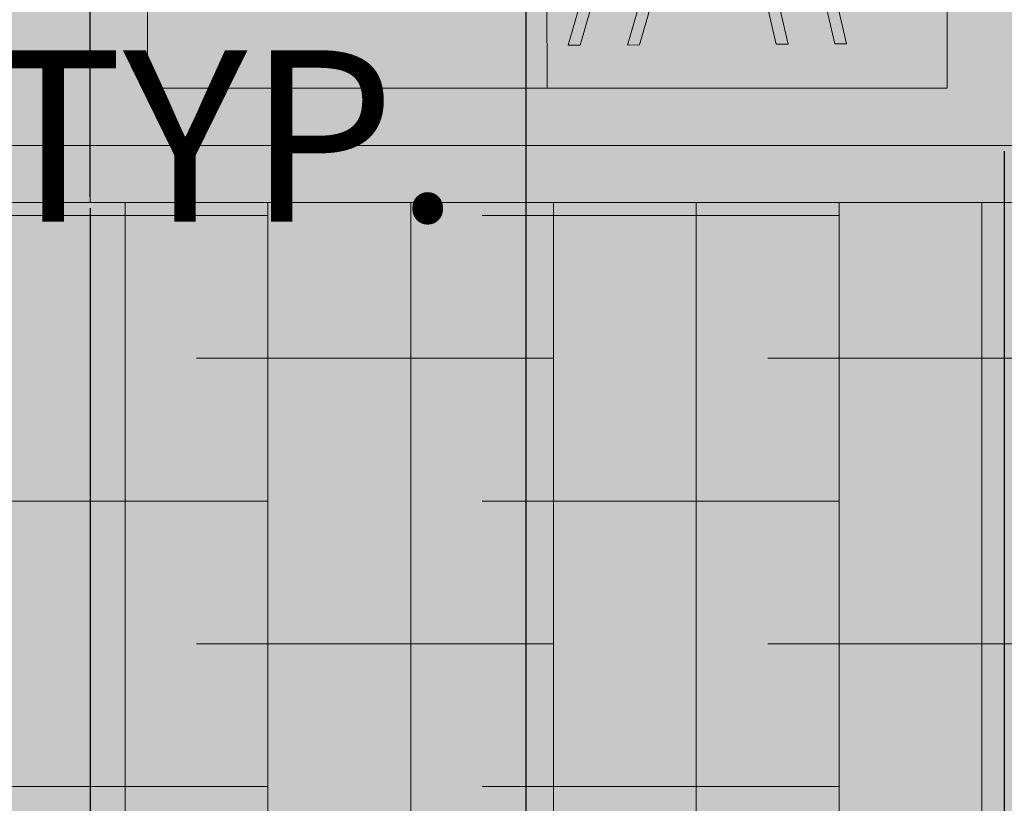
# Model space of a CAD drawing. Units: millimetres. Extents: x 11032 to 26788, y 3406 to 24505.
# Tile 5 of 78: x 16283 to 17145, y 6736 to 7421. Entities that reach past the tile are written whole.
import ezdxf

# ---------------------------------------------------------------- set-up
doc = ezdxf.new("R2010")
doc.units = ezdxf.units.MM
doc.header["$MEASUREMENT"] = 0
for name, color, linetype, lineweight in [('A-ANNO-DIMS', 2, 'Continuous', 18), ('A-FURN', 8, 'Continuous', 13), ('A-FURN-PATT', 8, 'Continuous', 13), ('A-GLAZ', 250, 'Continuous', 20), ('A-WALL-INTR', 8, 'Continuous', 18), ('A-WALL-PLIN-PATT', 253, 'Continuous', 13)]:
    doc.layers.add(name, color=color, linetype=linetype, lineweight=lineweight)
doc.layers.add('A-GLAZ-FRAM-PATT', color=250, linetype='Continuous', lineweight=13, true_color=0x262627)
doc.layers.add('A-WALL-INTR-PATT', color=251, linetype='Continuous', lineweight=13, true_color=0x6c6b6a)
doc.styles.get("Standard").update_dxf_attribs({"font": 'arial.ttf'})
doc.dimstyles.get("Standard").update_dxf_attribs({"dimtxt": 150, "dimasz": 100, "dimexe": 10, "dimexo": 5, "dimgap": 5, "dimtad": 0, "dimtih": 1, "dimtoh": 1, "dimdec": 0, "dimzin": 0, "dimdsep": 46, "dimtxsty": 'Standard', "dimcen": 0.09, "dimadec": 0, "dimazin": 0, "dimtfac": 1, "dimtdec": 0, "dimtofl": 0, "dimtmove": 0, "dimatfit": 3, "dimfxl": 1, "dimtolj": 1, "dimtzin": 0, "dimarcsym": 0})

# ---------------------------------------------------------------- blocks, each defined once
blk = doc.blocks.new('DINING-CHAIR-ELEV')
blk.add_line((228.68, 123.43), (51.04, 132.61))
for points in [[(0, 379.55), (49.45, 435.94), (114.12, 434.53)], [(61.18, 132.09), (30.79, 1.16), (20.53, 1.21), (59.55, 169.26), (0, 379.55), (61.9, 377.89)], [(111.9, 129.47), (82.06, 0.91), (71.8, 0.96), (101.76, 129.99)], [(165.28, 126.71), (201.76, 0.31), (212.19, 0.26), (175.85, 126.16)]]:
    blk.add_lwpolyline(points)
for points in [[(218.11, 123.98), (253.88, 0.05), (264.3, 0), (228.68, 123.43), (238.32, 182.18, 0.148451), (167.47, 178.33), (96.61, 174.48, 0.097012), (61.9, 377.89), (114.12, 434.53, -0.154833), (167.82, 178.46)], [(132.04, 176.4, 0.156877), (88.01, 406.21), (24.72, 407.74)]]:
    blk.add_lwpolyline(points, format="xyb")
blk = doc.blocks.new('*D16')
at = {"layer": 'A-ANNO-DIMS', "color": 0, "lineweight": -2, "transparency": 16777216}
for p, q in [((15741.74, 7821.05), (15812.13, 7821.05)), ((15802.13, 7721.05), (15802.13, 7685.69)), ((15802.13, 7485.11), (15802.13, 7520.47)), ((15741.74, 7385.11), (15812.13, 7385.11))]:
    blk.add_line(p, q, dxfattribs=at)
at = {"layer": 'A-ANNO-DIMS', "color": 0, "transparency": 16777216}
for points in [[(15785.47, 7721.05), (15818.8, 7721.05), (15802.13, 7821.05)], [(15785.47, 7485.11), (15818.8, 7485.11), (15802.13, 7385.11)]]:
    blk.add_solid(points, dxfattribs=at)
at = {"layer": 'Defpoints', "color": 0, "transparency": 16777216}
for p in [(15736.74, 7821.05), (15802.13, 7821.05), (15736.74, 7385.11)]:
    blk.add_point(p, dxfattribs=at)
at = {"layer": 'A-ANNO-DIMS', "color": 0, "transparency": 16777216, "insert": (15802.13, 7603.08), "char_height": 150, "attachment_point": 5}
blk.add_mtext('\\A1;CHAIR 436 TYP.', dxfattribs=at)
blk = doc.blocks.new('*D17')
at = {"layer": 'A-ANNO-DIMS', "color": 0, "lineweight": -2, "transparency": 16777216}
for p, q in [((15472.44, 7380.11), (15472.44, 7309.72)), ((15736.74, 7380.11), (15736.74, 7309.72)), ((15572.44, 7319.72), (15636.74, 7319.72)), ((15736.74, 7319.72), (15836.74, 7319.72))]:
    blk.add_line(p, q, dxfattribs=at)
at = {"layer": 'A-ANNO-DIMS', "color": 0, "transparency": 16777216}
for points in [[(15572.44, 7336.38), (15572.44, 7303.05), (15472.44, 7319.72)], [(15636.74, 7336.38), (15636.74, 7303.05), (15736.74, 7319.72)]]:
    blk.add_solid(points, dxfattribs=at)
at = {"layer": 'Defpoints', "color": 0, "transparency": 16777216}
for p in [(15472.44, 7385.11), (15736.74, 7385.11), (15736.74, 7319.72)]:
    blk.add_point(p, dxfattribs=at)
at = {"layer": 'A-ANNO-DIMS', "color": 0, "transparency": 16777216, "insert": (16266.37, 7319.72), "char_height": 150, "attachment_point": 5}
blk.add_mtext('\\A1;264 TYP.', dxfattribs=at)
blk = doc.blocks.new('*D36')
at = {"layer": 'A-ANNO-DIMS', "color": 0, "lineweight": -2, "transparency": 16777216}
for p, q in [((12301.26, 17115.89), (12301.26, 24416.86)), ((25397.4, 4466.4), (25397.4, 24416.86)), ((12401.26, 24406.86), (18569.2, 24406.86)), ((25297.4, 24406.86), (19129.47, 24406.86))]:
    blk.add_line(p, q, dxfattribs=at)
at = {"layer": 'A-ANNO-DIMS', "color": 0, "transparency": 16777216}
for points in [[(12401.26, 24423.52), (12401.26, 24390.19), (12301.26, 24406.86)], [(25297.4, 24423.52), (25297.4, 24390.19), (25397.4, 24406.86)]]:
    blk.add_solid(points, dxfattribs=at)
at = {"layer": 'Defpoints', "color": 0, "transparency": 16777216}
for p in [(25397.4, 24406.86), (12301.26, 17110.89), (25397.4, 4461.4)]:
    blk.add_point(p, dxfattribs=at)
at = {"layer": 'A-ANNO-DIMS', "color": 0, "transparency": 16777216, "insert": (18849.33, 24406.86), "char_height": 150, "attachment_point": 5}
blk.add_mtext('\\A1;13096', dxfattribs=at)
blk = doc.blocks.new('*D37')
at = {"layer": 'A-ANNO-DIMS', "color": 0, "lineweight": -2, "transparency": 16777216}
for p, q in [((18087.74, 23450.36), (11334.76, 23450.36)), ((11344.76, 23350.36), (11344.76, 14037.46)), ((11344.76, 4561.4), (11344.76, 13874.29)), ((12927.66, 4461.4), (11334.76, 4461.4))]:
    blk.add_line(p, q, dxfattribs=at)
at = {"layer": 'A-ANNO-DIMS', "color": 0, "transparency": 16777216}
for points in [[(11328.1, 23350.36), (11361.43, 23350.36), (11344.76, 23450.36)], [(11328.1, 4561.4), (11361.43, 4561.4), (11344.76, 4461.4)]]:
    blk.add_solid(points, dxfattribs=at)
at = {"layer": 'Defpoints', "color": 0, "transparency": 16777216}
for p in [(11344.76, 23450.36), (18092.74, 23450.36), (12932.66, 4461.4)]:
    blk.add_point(p, dxfattribs=at)
at = {"layer": 'A-ANNO-DIMS', "color": 0, "transparency": 16777216, "insert": (11344.76, 13955.88), "char_height": 150, "attachment_point": 5}
blk.add_mtext('\\A1;18989', dxfattribs=at)
blk = doc.blocks.new('*D49')
at = {"layer": 'A-ANNO-DIMS', "color": 0, "lineweight": -2, "transparency": 16777216}
for p, q in [((17953.45, 10206.41), (17953.45, 3494.9)), ((14996.4, 6406.4), (14996.4, 3494.9)), ((15096.4, 3504.9), (16244.67, 3504.9)), ((17853.45, 3504.9), (16705.18, 3504.9))]:
    blk.add_line(p, q, dxfattribs=at)
at = {"layer": 'A-ANNO-DIMS', "color": 0, "transparency": 16777216}
for points in [[(15096.4, 3521.57), (15096.4, 3488.23), (14996.4, 3504.9)], [(17853.45, 3521.57), (17853.45, 3488.23), (17953.45, 3504.9)]]:
    blk.add_solid(points, dxfattribs=at)
at = {"layer": 'Defpoints', "color": 0, "transparency": 16777216}
for p in [(17953.45, 10211.41), (14996.4, 6411.4), (17953.45, 3504.9)]:
    blk.add_point(p, dxfattribs=at)
at = {"layer": 'A-ANNO-DIMS', "color": 0, "transparency": 16777216, "insert": (16474.93, 3504.9), "char_height": 150, "attachment_point": 5}
blk.add_mtext('\\A1;2957', dxfattribs=at)
blk = doc.blocks.new('*D57')
at = {"layer": 'A-ANNO-DIMS', "color": 0, "lineweight": -2, "transparency": 16777216}
for p, q in [((14994.7, 7266.4), (14994.7, 24416.86)), ((20894.7, 7266.4), (20894.7, 24416.86)), ((15094.7, 24406.86), (17715.98, 24406.86)), ((20794.7, 24406.86), (18173.42, 24406.86))]:
    blk.add_line(p, q, dxfattribs=at)
at = {"layer": 'A-ANNO-DIMS', "color": 0, "transparency": 16777216}
for points in [[(15094.7, 24423.52), (15094.7, 24390.19), (14994.7, 24406.86)], [(20794.7, 24423.52), (20794.7, 24390.19), (20894.7, 24406.86)]]:
    blk.add_solid(points, dxfattribs=at)
at = {"layer": 'Defpoints', "color": 0, "transparency": 16777216}
for p in [(20894.7, 24406.86), (14994.7, 7261.4), (20894.7, 7261.4)]:
    blk.add_point(p, dxfattribs=at)
at = {"layer": 'A-ANNO-DIMS', "color": 0, "transparency": 16777216, "insert": (17944.7, 24406.86), "char_height": 150, "attachment_point": 5}
blk.add_mtext('\\A1;5900', dxfattribs=at)
blk = doc.blocks.new('*D60')
at = {"layer": 'A-ANNO-DIMS', "color": 0, "lineweight": -2, "transparency": 16777216}
for p, q in [((14994.7, 7266.4), (14994.7, 24416.86)), ((16344.7, 7266.4), (16344.7, 24416.86)), ((15094.7, 24406.86), (15448.04, 24406.86)), ((16244.7, 24406.86), (15891.36, 24406.86))]:
    blk.add_line(p, q, dxfattribs=at)
at = {"layer": 'A-ANNO-DIMS', "color": 0, "transparency": 16777216}
for points in [[(15094.7, 24423.52), (15094.7, 24390.19), (14994.7, 24406.86)], [(16244.7, 24423.52), (16244.7, 24390.19), (16344.7, 24406.86)]]:
    blk.add_solid(points, dxfattribs=at)
at = {"layer": 'Defpoints', "color": 0, "transparency": 16777216}
for p in [(16344.7, 24406.86), (14994.7, 7261.4), (16344.7, 7261.4)]:
    blk.add_point(p, dxfattribs=at)
at = {"layer": 'A-ANNO-DIMS', "color": 0, "transparency": 16777216, "insert": (15669.7, 24406.86), "char_height": 150, "attachment_point": 5}
blk.add_mtext('\\A1;1350', dxfattribs=at)
blk = doc.blocks.new('*D61')
at = {"layer": 'A-ANNO-DIMS', "color": 0, "lineweight": -2, "transparency": 16777216}
for p, q in [((17144.7, 7306.4), (17144.7, 3494.9)), ((16344.7, 7256.4), (16344.7, 3494.9)), ((16444.7, 3504.9), (16574.15, 3504.9)), ((17044.7, 3504.9), (16915.26, 3504.9))]:
    blk.add_line(p, q, dxfattribs=at)
at = {"layer": 'A-ANNO-DIMS', "color": 0, "transparency": 16777216}
for points in [[(16444.7, 3521.57), (16444.7, 3488.23), (16344.7, 3504.9)], [(17044.7, 3521.57), (17044.7, 3488.23), (17144.7, 3504.9)]]:
    blk.add_solid(points, dxfattribs=at)
at = {"layer": 'Defpoints', "color": 0, "transparency": 16777216}
for p in [(17144.7, 7311.4), (16344.7, 7261.4), (17144.7, 3504.9)]:
    blk.add_point(p, dxfattribs=at)
at = {"layer": 'A-ANNO-DIMS', "color": 0, "transparency": 16777216, "insert": (16744.7, 3504.9), "char_height": 150, "attachment_point": 5}
blk.add_mtext('\\A1;800', dxfattribs=at)
blk = doc.blocks.new('*D62')
at = {"layer": 'A-ANNO-DIMS', "color": 0, "lineweight": -2, "transparency": 16777216}
for p, q in [((17144.7, 7306.4), (17144.7, 3494.9)), ((17944.7, 7256.4), (17944.7, 3494.9)), ((17244.7, 3504.9), (17374.15, 3504.9)), ((17844.7, 3504.9), (17715.26, 3504.9))]:
    blk.add_line(p, q, dxfattribs=at)
at = {"layer": 'A-ANNO-DIMS', "color": 0, "transparency": 16777216}
for points in [[(17244.7, 3521.57), (17244.7, 3488.23), (17144.7, 3504.9)], [(17844.7, 3521.57), (17844.7, 3488.23), (17944.7, 3504.9)]]:
    blk.add_solid(points, dxfattribs=at)
at = {"layer": 'Defpoints', "color": 0, "transparency": 16777216}
for p in [(17144.7, 7311.4), (17944.7, 7261.4), (17944.7, 3504.9)]:
    blk.add_point(p, dxfattribs=at)
at = {"layer": 'A-ANNO-DIMS', "color": 0, "transparency": 16777216, "insert": (17544.7, 3504.9), "char_height": 150, "attachment_point": 5}
blk.add_mtext('\\A1;800', dxfattribs=at)
blk = doc.blocks.new('*D66')
at = {"layer": 'A-ANNO-DIMS', "color": 0, "lineweight": -2, "transparency": 16777216}
for p, q in [((16725.95, 10296.02), (16725.95, 3494.9)), ((19150.95, 10296.02), (19150.95, 3494.9)), ((16825.95, 3504.9), (17707.63, 3504.9)), ((19050.95, 3504.9), (18169.27, 3504.9))]:
    blk.add_line(p, q, dxfattribs=at)
at = {"layer": 'A-ANNO-DIMS', "color": 0, "transparency": 16777216}
for points in [[(16825.95, 3521.57), (16825.95, 3488.23), (16725.95, 3504.9)], [(19050.95, 3521.57), (19050.95, 3488.23), (19150.95, 3504.9)]]:
    blk.add_solid(points, dxfattribs=at)
at = {"layer": 'Defpoints', "color": 0, "transparency": 16777216}
for p in [(16725.95, 10301.02), (19150.95, 10301.02), (19150.95, 3504.9)]:
    blk.add_point(p, dxfattribs=at)
at = {"layer": 'A-ANNO-DIMS', "color": 0, "transparency": 16777216, "insert": (17938.45, 3504.9), "char_height": 150, "attachment_point": 5}
blk.add_mtext('\\A1;2425', dxfattribs=at)
blk = doc.blocks.new('*D69')
at = {"layer": 'A-ANNO-DIMS', "color": 0, "lineweight": -2, "transparency": 16777216}
for p, q in [((13956.97, 9937.95), (14056.97, 9937.95)), ((14056.97, 9937.95), (15432.5, 8990.95)), ((17944.61, 7261.4), (17944.79, 7261.4)), ((17944.7, 7261.31), (17944.7, 7261.49))]:
    blk.add_line(p, q, dxfattribs=at)
at = {"layer": 'A-ANNO-DIMS', "color": 0, "transparency": 16777216}
blk.add_solid([(15441.95, 9004.68), (15423.05, 8977.22), (15514.87, 8934.24)], dxfattribs=at)
at = {"layer": 'Defpoints', "color": 0, "transparency": 16777216}
for p in [(15514.87, 8934.24), (17944.7, 7261.4)]:
    blk.add_point(p, dxfattribs=at)
at = {"layer": 'A-ANNO-DIMS', "color": 0, "transparency": 16777216, "insert": (13494.04, 9937.95), "char_height": 150, "attachment_point": 5}
blk.add_mtext('\\A1;2X R2950', dxfattribs=at)

msp = doc.modelspace()

# ---------------------------------------------------------------- hatches: boundary and pattern name
at = {"layer": 'A-FURN-PATT'}
h = msp.add_hatch(color=256, dxfattribs=at)
h.set_gradient(color1=(82, 15, 16), color2=(153, 0, 38), name='CURVED')
h.paths.add_polyline_path([(16952.125, 8119), (16926.017, 8147.32, 0.1568775), (16881.989, 7917.509), (16917.415, 7915.583, -0.0970121)], flags=0)
h.paths.add_polyline_path([(16899.908, 8175.64), (16964.58, 8177.046), (17014.03, 8120.657), (16954.484, 7910.365), (16972.017, 7834.84), (16977.75, 7834.965), (17027.199, 7778.576), (16967.653, 7568.284), (17006.665, 7400.238), (16996.411, 7400.187), (16966.016, 7531.114), (16925.439, 7529.018), (16955.395, 7399.983), (16945.141, 7399.932), (16915.295, 7528.494), (16861.916, 7525.736), (16825.435, 7399.337), (16815.012, 7399.285), (16851.35, 7525.19), (16809.087, 7523.007), (16773.319, 7399.078), (16762.896, 7399.026), (16798.521, 7522.461), (16788.882, 7581.207, -0.1476694), (16859.382, 7577.482, -0.1528132), (16911.41, 7830.579), (16902.125, 7870.575), (16848.746, 7867.817), (16830.506, 7804.617), (16830.506, 7793.515), (16827.302, 7793.515), (16812.265, 7741.418), (16801.842, 7741.366), (16816.893, 7793.515), (16775.261, 7793.515), (16760.15, 7741.159), (16749.727, 7741.107), (16764.853, 7793.515), (16650.704, 7793.515), (16662.994, 7750.932), (16652.571, 7750.983), (16640.296, 7793.515), (16598.663, 7793.515), (16610.879, 7751.191), (16600.455, 7751.242), (16588.255, 7793.515), (16490.425, 7793.515), (16480.749, 7751.837), (16470.495, 7751.888), (16480.159, 7793.515), (16443.833, 7793.515, -0.1094051), (16465.746, 7607.731, -0.1476694), (16536.246, 7611.456), (16526.606, 7552.71), (16562.232, 7429.275), (16551.809, 7429.327), (16516.041, 7553.255), (16473.778, 7555.439), (16510.116, 7429.534), (16499.693, 7429.586), (16463.212, 7555.985), (16409.833, 7558.743), (16379.987, 7430.181), (16369.733, 7430.232), (16394.704, 7537.793), (16394.704, 7559.524), (16359.112, 7561.363), (16328.717, 7430.435), (16318.463, 7430.486), (16344.704, 7543.521), (16344.704, 7643.635), (16302.264, 7793.515), (16205.738, 7793.515), (16227.021, 7719.773), (16216.598, 7719.825), (16195.329, 7793.515), (16153.697, 7793.515), (16174.905, 7720.032), (16164.482, 7720.084), (16143.289, 7793.515), (15844.423, 7793.515), (15844.423, 7804.617), (16140.084, 7804.617), (16128.001, 7846.483), (16191.395, 7843.208), (16201.035, 7901.954, 0.1484508), (16130.184, 7898.102), (16059.333, 7894.25, 0.0970121), (16024.622, 8097.666), (16076.839, 8154.307, -0.1548334), (16130.535, 7898.229, -0.1476694), (16201.035, 7901.954), (16191.395, 7843.208), (16202.533, 7804.617), (16299.12, 7804.617), (16297.929, 7808.825), (16347.378, 7865.214), (16412.05, 7863.808, -0.0295496), (16434.494, 7817.915), (16458.237, 7920.19), (16398.691, 8130.481), (16448.141, 8186.871), (16512.813, 8185.465, -0.1548334), (16566.508, 7929.387, -0.1476694), (16637.008, 7933.112), (16627.369, 7874.366), (16647.499, 7804.617), (16742.939, 7804.617), (16741.107, 8264.696), (17994.704, 8264.696), (17994.704, 7796.661), (18112.02, 7796.661), (18134.447, 7874.366), (18124.807, 7933.112, -0.1476694), (18195.307, 7929.387, -0.1548334), (18249.003, 8185.465), (18313.675, 8186.871), (18363.124, 8130.481), (18303.578, 7920.19), (18311.087, 7887.847, -0.0273017), (18332.016, 7930.161), (18396.688, 7931.567), (18446.137, 7875.177), (18423.905, 7796.661), (18470.25, 7796.661), (18470.25, 7785.559), (18420.761, 7785.559), (18386.591, 7664.886), (18425.604, 7496.839), (18415.35, 7496.788), (18384.955, 7627.716), (18344.377, 7625.62), (18374.333, 7496.584), (18364.079, 7496.533), (18334.233, 7625.095), (18280.854, 7622.338), (18244.373, 7495.938), (18233.95, 7495.887), (18270.288, 7621.792), (18228.026, 7619.608), (18192.257, 7495.679), (18181.834, 7495.628), (18217.46, 7619.062), (18207.82, 7677.808, -0.1476694), (18278.32, 7674.083, -0.0514181), (18278.516, 7762.821), (18273.237, 7785.559), (18171.265, 7785.559), (18161.36, 7751.242), (18150.937, 7751.191), (18160.856, 7785.559), (18119.224, 7785.559), (18109.244, 7750.983), (18098.821, 7750.932), (18108.815, 7785.559), (17852.794, 7785.559), (17866.18, 7739.181), (17855.756, 7739.233), (17842.386, 7785.559), (17800.753, 7785.559), (17814.064, 7739.44), (17803.641, 7739.492), (17790.345, 7785.559), (17694.491, 7785.559), (17685.986, 7748.922, -0.0882745), (17728.687, 7746.171), (17719.047, 7687.425), (17754.673, 7563.99), (17744.25, 7564.042), (17708.482, 7687.971), (17666.219, 7690.154), (17702.557, 7564.249), (17692.134, 7564.301), (17655.653, 7690.7), (17602.274, 7693.458), (17572.428, 7564.896), (17562.174, 7564.947), (17592.13, 7693.982), (17551.553, 7696.078), (17521.158, 7565.151), (17510.903, 7565.202), (17549.916, 7733.248), (17535.103, 7785.559), (17484.167, 7785.559), (17484.167, 7796.661), (17531.96, 7796.661), (17490.37, 7943.54), (17539.819, 7999.929), (17604.491, 7998.523, -0.0802486), (17652.289, 7869.096), (17661.422, 7908.439), (17601.876, 8118.731), (17651.326, 8175.12), (17715.998, 8173.714, -0.1548334), (17769.694, 7917.637, -0.1476694), (17840.194, 7921.361), (17830.554, 7862.615), (17849.59, 7796.661), (17894.704, 7796.661), (17894.704, 8239.696), (16741.207, 8239.696), (16742.939, 7804.617), (16768.057, 7804.617), (16785.352, 7864.542), (16775.713, 7923.288, -0.1476694), (16846.212, 7919.563, -0.1548334)], flags=17)
h.paths.add_polyline_path([(16899.908, 8175.64), (16964.58, 8177.046), (17014.03, 8120.657), (16954.484, 7910.365), (16993.496, 7742.318), (16983.242, 7742.267), (16952.847, 7873.195), (16912.27, 7871.099), (16942.225, 7742.064), (16931.971, 7742.013), (16902.125, 7870.575), (16848.746, 7867.817), (16812.265, 7741.418), (16801.842, 7741.366), (16838.181, 7867.271), (16795.918, 7865.087), (16760.15, 7741.159), (16749.727, 7741.107), (16785.352, 7864.542), (16775.713, 7923.288, -0.1476694), (16846.212, 7919.563, -0.1548334)], flags=0)
h.paths.add_polyline_path([(16899.908, 8175.64), (16964.58, 8177.046), (17014.03, 8120.657), (16954.484, 7910.365), (16972.017, 7834.84), (16977.75, 7834.965), (17027.199, 7778.576), (16967.653, 7568.284), (17006.665, 7400.238), (16996.411, 7400.187), (16966.016, 7531.114), (16925.439, 7529.018), (16955.395, 7399.983), (16945.141, 7399.932), (16915.295, 7528.494), (16861.916, 7525.736), (16825.435, 7399.337), (16815.012, 7399.285), (16851.35, 7525.19), (16809.087, 7523.007), (16773.319, 7399.078), (16762.896, 7399.026), (16798.521, 7522.461), (16788.882, 7581.207, -0.1476694), (16859.382, 7577.482, -0.1528132), (16911.41, 7830.579), (16902.125, 7870.575), (16848.746, 7867.817), (16830.506, 7804.617), (16830.506, 7793.515), (16827.302, 7793.515), (16812.265, 7741.418), (16801.842, 7741.366), (16816.893, 7793.515), (16775.261, 7793.515), (16760.15, 7741.159), (16749.727, 7741.107), (16764.853, 7793.515), (16650.704, 7793.515), (16662.994, 7750.932), (16652.571, 7750.983), (16640.296, 7793.515), (16598.663, 7793.515), (16610.879, 7751.191), (16600.455, 7751.242), (16588.255, 7793.515), (16490.425, 7793.515), (16480.749, 7751.837), (16470.495, 7751.888), (16480.159, 7793.515), (16443.833, 7793.515, -0.1094051), (16465.746, 7607.731, -0.1476694), (16536.246, 7611.456), (16526.606, 7552.71), (16562.232, 7429.275), (16551.809, 7429.327), (16516.041, 7553.255), (16473.778, 7555.439), (16510.116, 7429.534), (16499.693, 7429.586), (16463.212, 7555.985), (16409.833, 7558.743), (16379.987, 7430.181), (16369.733, 7430.232), (16394.704, 7537.793), (16394.704, 7559.524), (16359.112, 7561.363), (16328.717, 7430.435), (16318.463, 7430.486), (16344.704, 7543.521), (16344.704, 7643.635), (16302.264, 7793.515), (16205.738, 7793.515), (16227.021, 7719.773), (16216.598, 7719.825), (16195.329, 7793.515), (16153.697, 7793.515), (16174.905, 7720.032), (16164.482, 7720.084), (16143.289, 7793.515), (15844.423, 7793.515), (15844.423, 7804.617), (16140.084, 7804.617), (16128.001, 7846.483), (16191.395, 7843.208), (16201.035, 7901.954, 0.1484508), (16130.184, 7898.102), (16059.333, 7894.25, 0.0970121), (16024.622, 8097.666), (16076.839, 8154.307, -0.1548334), (16130.535, 7898.229, -0.1476694), (16201.035, 7901.954), (16191.395, 7843.208), (16202.533, 7804.617), (16299.12, 7804.617), (16297.929, 7808.825), (16347.378, 7865.214), (16412.05, 7863.808, -0.0295496), (16434.494, 7817.915), (16458.237, 7920.19), (16398.691, 8130.481), (16448.141, 8186.871), (16512.813, 8185.465, -0.1548334), (16566.508, 7929.387, -0.1476694), (16637.008, 7933.112), (16627.369, 7874.366), (16647.499, 7804.617), (16742.939, 7804.617), (16741.207, 8239.696), (16741.107, 8264.696), (17994.704, 8264.696), (17994.704, 7796.661), (18112.02, 7796.661), (18134.447, 7874.366), (18124.807, 7933.112, -0.1476694), (18195.307, 7929.387, -0.1548334), (18249.003, 8185.465), (18313.675, 8186.871), (18363.124, 8130.481), (18303.578, 7920.19), (18311.087, 7887.847, -0.0273017), (18332.016, 7930.161), (18396.688, 7931.567), (18446.137, 7875.177), (18423.905, 7796.661), (18470.25, 7796.661), (18470.25, 7785.559), (18420.761, 7785.559), (18386.591, 7664.886), (18425.604, 7496.839), (18415.35, 7496.788), (18384.955, 7627.716), (18344.377, 7625.62), (18374.333, 7496.584), (18364.079, 7496.533), (18334.233, 7625.095), (18280.854, 7622.338), (18244.373, 7495.938), (18233.95, 7495.887), (18270.288, 7621.792), (18228.026, 7619.608), (18192.257, 7495.679), (18181.834, 7495.628), (18217.46, 7619.062), (18207.82, 7677.808, -0.1476694), (18278.32, 7674.083, -0.0514181), (18278.516, 7762.821), (18273.237, 7785.559), (18171.265, 7785.559), (18161.36, 7751.242), (18150.937, 7751.191), (18160.856, 7785.559), (18119.224, 7785.559), (18109.244, 7750.983), (18098.821, 7750.932), (18108.815, 7785.559), (17852.794, 7785.559), (17866.18, 7739.181), (17855.756, 7739.233), (17842.386, 7785.559), (17800.753, 7785.559), (17814.064, 7739.44), (17803.641, 7739.492), (17790.345, 7785.559), (17694.491, 7785.559), (17685.986, 7748.922, -0.0882745), (17728.687, 7746.171), (17719.047, 7687.425), (17754.673, 7563.99), (17744.25, 7564.042), (17708.482, 7687.971), (17666.219, 7690.154), (17702.557, 7564.249), (17692.134, 7564.301), (17655.653, 7690.7), (17602.274, 7693.458), (17572.428, 7564.896), (17562.174, 7564.947), (17592.13, 7693.982), (17551.553, 7696.078), (17521.158, 7565.151), (17510.903, 7565.202), (17549.916, 7733.248), (17535.103, 7785.559), (17484.167, 7785.559), (17484.167, 7796.661), (17531.96, 7796.661), (17490.37, 7943.54), (17539.819, 7999.929), (17604.491, 7998.523, -0.0802486), (17652.289, 7869.096), (17661.422, 7908.439), (17601.876, 8118.731), (17651.326, 8175.12), (17715.998, 8173.714, -0.1548334), (17769.694, 7917.637, -0.1476694), (17840.194, 7921.361), (17830.554, 7862.615), (17849.59, 7796.661), (17894.704, 7796.661), (17894.704, 8239.696), (16741.207, 8239.696), (16742.939, 7804.617), (16768.057, 7804.617), (16785.352, 7864.542), (16775.713, 7923.288, -0.1476694), (16846.212, 7919.563, -0.1548334)], flags=17)
h = msp.add_hatch(color=256, dxfattribs=at)
h.set_gradient(color1=(82, 15, 16), color2=(153, 0, 38), name='CURVED')
h.paths.add_polyline_path([(16913.077, 7833.559), (16977.75, 7834.965), (17027.199, 7778.576), (16967.653, 7568.284), (17006.665, 7400.238), (16996.411, 7400.187), (16966.016, 7531.114), (16925.439, 7529.018), (16955.395, 7399.983), (16945.141, 7399.932), (16915.295, 7528.494), (16861.916, 7525.736), (16825.435, 7399.337), (16815.012, 7399.285), (16851.35, 7525.19), (16809.087, 7523.007), (16773.319, 7399.078), (16762.896, 7399.026), (16798.521, 7522.461), (16788.882, 7581.207, -0.1476694), (16859.382, 7577.482, -0.1548334)])
h.paths.add_polyline_path([(16881.989, 7917.509), (16917.415, 7915.583, -0.0970121), (16952.125, 8119), (16926.017, 8147.32, 0.1568775)])
at = {"layer": 'A-GLAZ-FRAM-PATT'}
h = msp.add_hatch(color=256, dxfattribs=at)
h.paths.add_polyline_path([(17944.704, 7311.399), (16344.704, 7311.399), (16344.704, 7261.399), (17944.704, 7261.399)], flags=17)
h.paths.add_polyline_path([(16344.704, 7311.399), (15045.135, 7311.399, -0.9829047), (20844.273, 7311.399), (19544.704, 7311.399), (19544.704, 7261.399), (20894.704, 7261.399, 0.5148441), (16985.951, 10051.255, 0.3202679), (14994.704, 7261.399), (16344.704, 7261.399)])
h.paths.add_polyline_path([(18744.704, 7311.399), (17944.704, 7311.399), (17944.704, 7261.399), (18744.704, 7261.399)], flags=17)
h.paths.add_polyline_path([(19544.704, 7311.399), (18744.704, 7311.399), (18744.704, 7261.399), (19544.704, 7261.399)], flags=17)
h.paths.add_polyline_path([(18694.704, 7361.399), (17994.704, 7361.399), (17994.704, 7311.399), (18694.704, 7311.399)], flags=17)
h.paths.add_polyline_path([(18744.704, 7361.399), (18694.704, 7361.399), (18694.704, 7311.399), (18744.704, 7311.399)], flags=17)
h.paths.add_polyline_path([(17194.704, 7361.399), (17144.704, 7361.399), (17144.704, 7311.399), (17194.704, 7311.399)], flags=17)
h.paths.add_polyline_path([(17431.432, 7361.399), (17194.704, 7361.399), (17194.704, 7311.399), (17431.699, 7311.399)], flags=17)
h.paths.add_polyline_path([(17894.704, 7361.399), (17431.432, 7361.399), (17431.699, 7311.399), (17894.704, 7311.399)], flags=17)
h.paths.add_polyline_path([(17944.704, 7361.399), (17894.704, 7361.399), (17894.704, 7311.399), (17944.704, 7311.399)], flags=17)
h.paths.add_polyline_path([(17994.704, 7361.399), (17944.704, 7361.399), (17944.704, 7311.399), (17994.704, 7311.399)], flags=17)
h = msp.add_hatch(color=256, dxfattribs=at)
h.paths.add_polyline_path([(16734.609, 9896.863, 0.0333754), (16394.704, 9712.419), (16394.704, 7804.617), (16431.407, 7804.617), (16458.237, 7920.19), (16398.691, 8130.481), (16448.141, 8186.871), (16512.813, 8185.465, -0.1548334), (16566.508, 7929.387, -0.1476694), (16637.008, 7933.112), (16627.369, 7874.366), (16647.499, 7804.617), (16742.939, 7804.617)])
h.paths.add_polyline_path([(17094.704, 9961.399), (16886.403, 9961.399, 0.0142221), (16734.609, 9896.863), (16741.107, 8264.696), (17094.704, 8264.696)])
h.paths.add_polyline_path([(17417.202, 10027.292), (17194.704, 10011.399), (17194.704, 8264.696), (17426.61, 8264.696)])
h.paths.add_polyline_path([(17144.704, 8239.696), (17094.704, 8239.696), (17094.704, 7361.399), (16394.704, 7361.399), (16394.704, 7493.572), (16379.987, 7430.181), (16369.733, 7430.232), (16394.704, 7537.793), (16394.704, 7559.524), (16359.112, 7561.363), (16344.704, 7499.3), (16344.704, 7311.399), (17144.704, 7311.399)])
h.paths.add_polyline_path([(17194.704, 8239.696), (17144.704, 8239.696), (17144.704, 7361.399), (17194.704, 7361.399)])
at = {"layer": 'A-WALL-INTR-PATT'}
h = msp.add_hatch(color=256, dxfattribs=at)
h.paths.add_polyline_path([(15302.659, 8457.059, 0.0281002), (15185.248, 8153.253), (15233.282, 7717.599), (15314.374, 7311.399), (15467.334, 7311.399), (15381.661, 7740.545)])
h.paths.add_polyline_path([(16344.704, 7543.521), (16344.704, 7643.635), (16302.264, 7793.515), (16205.738, 7793.515), (16227.021, 7719.773), (16216.598, 7719.825), (16195.329, 7793.515), (16153.697, 7793.515), (16174.905, 7720.032), (16164.482, 7720.084), (16143.289, 7793.515), (16061.685, 7793.515), (16051.641, 7750.248, -0.0167144), (16059.629, 7748.571), (16049.99, 7689.825), (16085.615, 7566.39), (16075.192, 7566.442), (16039.424, 7690.371), (15997.161, 7692.554), (16033.5, 7566.649), (16023.077, 7566.701), (15986.595, 7693.1), (15933.216, 7695.858), (15903.371, 7567.296), (15893.116, 7567.347), (15923.072, 7696.382), (15882.495, 7698.478), (15852.409, 7568.882), (15877.716, 7481.201), (15867.293, 7481.253), (15844.553, 7560.041), (15844.691, 7311.399), (16344.704, 7311.399), (16344.704, 7499.3), (16328.717, 7430.435), (16318.463, 7430.486)])
h.paths.add_polyline_path([(16742.983, 7793.515), (16650.704, 7793.515), (16662.994, 7750.932), (16652.571, 7750.983), (16640.296, 7793.515), (16598.663, 7793.515), (16610.879, 7751.191), (16600.455, 7751.242), (16588.255, 7793.515), (16490.425, 7793.515), (16480.749, 7751.837), (16470.495, 7751.888), (16480.159, 7793.515), (16443.833, 7793.515, -0.1094051), (16465.746, 7607.731, -0.1476694), (16536.246, 7611.456), (16526.606, 7552.71), (16562.232, 7429.275), (16551.809, 7429.327), (16516.041, 7553.255), (16473.778, 7555.439), (16510.116, 7429.534), (16499.693, 7429.586), (16463.212, 7555.985), (16409.833, 7558.743), (16394.704, 7493.572), (16394.704, 7361.399), (16744.704, 7361.399)])
h.paths.add_polyline_path([(17094.704, 8239.696), (16741.207, 8239.696), (16742.939, 7804.617), (16768.057, 7804.617), (16785.352, 7864.542), (16775.713, 7923.288, -0.1476694), (16846.212, 7919.563, -0.1548334), (16899.908, 8175.64), (16964.58, 8177.046), (17014.03, 8120.657), (16954.484, 7910.365), (16972.017, 7834.84), (16977.75, 7834.965), (17027.199, 7778.576), (16967.653, 7568.284), (17006.665, 7400.238), (16996.411, 7400.187), (16966.016, 7531.114), (16925.439, 7529.018), (16955.395, 7399.983), (16945.141, 7399.932), (16915.295, 7528.494), (16861.916, 7525.736), (16825.435, 7399.337), (16815.012, 7399.285), (16851.35, 7525.19), (16809.087, 7523.007), (16773.319, 7399.078), (16762.896, 7399.026), (16798.521, 7522.461), (16788.882, 7581.207, -0.1476694), (16859.382, 7577.482, -0.1528132), (16911.41, 7830.579), (16902.125, 7870.575), (16848.746, 7867.817), (16830.506, 7804.617), (16830.506, 7793.515), (16827.302, 7793.515), (16812.265, 7741.418), (16801.842, 7741.366), (16816.893, 7793.515), (16775.261, 7793.515), (16760.15, 7741.159), (16749.727, 7741.107), (16764.853, 7793.515), (16742.983, 7793.515), (16744.704, 7361.399), (17094.704, 7361.399)])
h.paths.add_polyline_path([(18950.929, 7931.023), (19015.601, 7932.429), (19065.05, 7876.04), (19005.504, 7665.748), (19014.012, 7629.102, -0.129191), (19069.892, 7841.762), (19134.564, 7843.167), (19168.958, 7803.946), (19202.145, 7841.791), (19246.92, 7840.817), (19212.932, 7960.847), (19262.382, 8017.236), (19327.054, 8015.831, -0.134919), (19382.824, 7793.43), (19562.845, 7793.43, -0.1257757), (19618.686, 8000.275), (19683.358, 8001.68), (19732.808, 7945.291), (19689.807, 7793.43), (19753.644, 7793.43, -0.0966843), (19805.964, 7950.707), (19870.637, 7952.112), (19920.086, 7895.723), (19891.121, 7793.43), (20039.255, 7793.43, -0.0897865), (20089.9, 7938.993), (20154.572, 7940.399), (20204.021, 7884.01), (20144.475, 7673.718), (20152.983, 7637.072, -0.1476694), (20223.483, 7633.347, -0.1548334), (20277.178, 7889.425), (20341.85, 7890.831), (20391.3, 7834.441), (20331.754, 7624.15), (20370.766, 7456.103), (20360.512, 7456.052), (20330.117, 7586.98), (20289.54, 7584.884), (20319.496, 7455.848), (20309.241, 7455.797), (20279.396, 7584.359), (20226.017, 7581.602), (20189.536, 7455.202), (20179.112, 7455.151), (20215.451, 7581.056), (20173.188, 7578.872), (20169.478, 7566.018), (20183.488, 7505.671), (20173.234, 7505.62), (20163.789, 7546.305), (20137.42, 7454.943), (20126.997, 7454.892), (20159.149, 7566.291), (20142.839, 7636.548), (20102.261, 7634.452), (20132.217, 7505.417), (20121.963, 7505.366), (20092.117, 7633.928), (20038.738, 7631.17), (20002.257, 7504.771), (19991.834, 7504.719), (20028.172, 7630.624), (19985.91, 7628.44), (19950.141, 7504.512), (19939.718, 7504.46), (19975.344, 7627.895), (19965.704, 7686.641, -0.1476694), (20036.204, 7682.916, -0.0576487), (20037.659, 7782.328), (19887.977, 7782.328), (19860.54, 7685.431), (19899.552, 7517.385), (19889.298, 7517.334), (19858.903, 7648.261), (19818.326, 7646.165), (19848.282, 7517.13), (19838.028, 7517.079), (19808.182, 7645.641), (19754.803, 7642.883), (19718.322, 7516.484), (19707.899, 7516.432), (19744.237, 7642.337), (19701.974, 7640.154), (19698.264, 7627.3), (19712.274, 7566.953), (19702.02, 7566.902), (19692.575, 7607.587), (19666.206, 7516.225), (19655.783, 7516.173), (19687.935, 7627.573), (19671.625, 7697.83), (19631.048, 7695.733), (19661.003, 7566.698), (19650.749, 7566.647), (19620.903, 7695.209), (19567.524, 7692.451), (19531.043, 7566.052), (19520.62, 7566), (19556.959, 7691.905), (19514.696, 7689.722), (19478.928, 7565.793), (19468.505, 7565.741), (19473, 7581.318), (19466.812, 7581.349), (19431.044, 7705.278), (19388.781, 7707.461), (19425.12, 7581.556), (19414.696, 7581.608), (19378.215, 7708.007), (19324.836, 7710.765), (19318.877, 7685.094, -0.0584523), (19320.513, 7584.307, -0.1476694), (19391.013, 7588.032), (19381.373, 7529.286), (19416.999, 7405.852), (19406.576, 7405.903), (19370.808, 7529.832), (19328.545, 7532.016), (19364.883, 7406.111), (19354.46, 7406.162), (19317.979, 7532.562), (19264.6, 7535.319), (19234.754, 7406.757), (19224.5, 7406.808), (19254.456, 7535.844), (19213.879, 7537.94), (19183.484, 7407.012), (19173.23, 7407.063), (19212.242, 7575.11), (19168.16, 7730.789), (19124.467, 7576.487), (19163.48, 7408.44), (19153.225, 7408.389), (19122.83, 7539.317), (19082.253, 7537.22), (19112.209, 7408.185), (19101.955, 7408.134), (19072.109, 7536.696), (19035.898, 7534.825), (19044.517, 7497.701), (19034.262, 7497.65), (19025.754, 7534.301), (19018.73, 7533.938), (18982.249, 7407.539), (18971.826, 7407.487), (19008.164, 7533.392), (18985.177, 7532.205), (18993.246, 7497.447), (18982.992, 7497.396), (18975.033, 7531.681), (18965.902, 7531.209), (18930.133, 7407.28), (18919.71, 7407.228), (18955.336, 7530.663), (18945.696, 7589.409, -0.0318483), (18960.996, 7592.142), (18953.146, 7625.958), (18899.767, 7623.2), (18863.286, 7496.801), (18852.863, 7496.749), (18889.201, 7622.654), (18846.938, 7620.47), (18811.17, 7496.542), (18800.747, 7496.49), (18836.373, 7619.924), (18826.733, 7678.67, -0.1476694), (18897.233, 7674.946, -0.1548334)], flags=16)
h = msp.add_hatch(color=256, dxfattribs=at)
h.set_gradient(color1=(254, 234, 185), color2=(254, 204, 102), name='CURVED')
h.paths.add_polyline_path([(15260.167, 7582.928), (15062.56, 7582.722, 0.023451), (15045.135, 7311.399), (15314.374, 7311.399)])
h.paths.add_polyline_path([(15413.095, 7583.087), (15260.167, 7582.928), (15314.374, 7311.399), (15467.334, 7311.399)])
h.paths.add_polyline_path([(15531.986, 7554.365), (15523.82, 7583.203), (15413.095, 7583.087), (15467.334, 7311.399), (15790.119, 7311.399), (15790.667, 7566.433), (15785.748, 7583.476), (15718.988, 7583.406), (15701.389, 7507.6), (15736.743, 7385.107), (15726.32, 7385.159), (15696.749, 7487.614), (15695.471, 7482.107), (15685.217, 7482.158), (15691.06, 7507.327), (15690.552, 7509.088), (15650.881, 7511.137), (15649.743, 7506.234), (15684.627, 7385.366), (15674.204, 7385.418), (15646.227, 7482.352), (15633.946, 7482.413), (15639.413, 7505.961), (15637.723, 7511.817), (15584.344, 7514.575), (15554.498, 7386.013), (15544.244, 7386.064), (15574.2, 7515.099), (15533.623, 7517.195), (15503.228, 7386.268), (15492.974, 7386.319)])
h.paths.add_polyline_path([(16344.704, 7499.3), (16328.717, 7430.435), (16318.463, 7430.486), (16344.704, 7543.521), (16344.704, 7584.059), (16080.595, 7583.783), (16085.615, 7566.39), (16075.192, 7566.442), (16070.19, 7583.773), (16028.57, 7583.729), (16033.5, 7566.649), (16023.077, 7566.701), (16018.165, 7583.718), (15907.156, 7583.603), (15903.371, 7567.296), (15893.116, 7567.347), (15896.888, 7583.592), (15855.814, 7583.549), (15852.409, 7568.882), (15877.716, 7481.201), (15867.293, 7481.253), (15844.553, 7560.041), (15844.691, 7311.399), (16344.704, 7311.399)])
h.paths.add_polyline_path([(15844.553, 7560.041), (15842.372, 7567.599), (15841.846, 7567.602), (15842.08, 7568.609), (15837.773, 7583.53), (15796.153, 7583.487), (15825.6, 7481.46), (15815.177, 7481.512), (15790.667, 7566.433), (15790.119, 7311.399), (15844.691, 7311.399)])
h.paths.add_polyline_path([(16394.704, 7493.572), (16379.987, 7430.181), (16369.733, 7430.232), (16394.704, 7537.793), (16394.704, 7559.524), (16359.112, 7561.363), (16344.704, 7499.3), (16344.704, 7311.399), (17144.704, 7311.399), (17144.704, 7584.893), (17094.704, 7584.841), (17094.704, 7361.399), (16394.704, 7361.399)])
h.paths.add_polyline_path([(17430.237, 7585.191), (17194.704, 7584.945), (17194.704, 7361.399), (17431.432, 7361.399)])
h.paths.add_polyline_path([(17894.704, 7585.675), (17748.458, 7585.522), (17754.673, 7563.99), (17744.25, 7564.042), (17738.053, 7585.511), (17696.433, 7585.468), (17702.557, 7564.249), (17692.134, 7564.301), (17686.028, 7585.457), (17577.175, 7585.344), (17572.428, 7564.896), (17562.174, 7564.947), (17566.907, 7585.333), (17525.833, 7585.29), (17521.158, 7565.151), (17510.903, 7565.202), (17515.565, 7585.28), (17430.237, 7585.191), (17431.432, 7361.399), (17894.704, 7361.399)])
h.paths.add_polyline_path([(18694.704, 7586.509), (18404.857, 7586.207), (18425.604, 7496.839), (18415.35, 7496.788), (18394.593, 7586.196), (18353.54, 7586.153), (18374.333, 7496.584), (18364.079, 7496.533), (18343.276, 7586.142), (18270.386, 7586.066), (18244.373, 7495.938), (18233.95, 7495.887), (18259.974, 7586.056), (18218.329, 7586.012), (18192.257, 7495.679), (18181.834, 7495.628), (18207.918, 7586.001), (17994.704, 7585.779), (17994.704, 7361.399), (18694.704, 7361.399)])
h.paths.add_polyline_path([(19317.979, 7532.562), (19264.6, 7535.319), (19234.754, 7406.757), (19224.5, 7406.808), (19254.456, 7535.844), (19213.879, 7537.94), (19183.484, 7407.012), (19173.23, 7407.063), (19212.242, 7575.11), (19208.862, 7587.045), (19127.433, 7586.96), (19124.467, 7576.487), (19163.48, 7408.44), (19153.225, 7408.389), (19122.83, 7539.317), (19082.253, 7537.22), (19112.209, 7408.185), (19101.955, 7408.134), (19072.109, 7536.696), (19035.898, 7534.825), (19044.517, 7497.701), (19034.262, 7497.65), (19025.754, 7534.301), (19018.73, 7533.938), (18982.249, 7407.539), (18971.826, 7407.487), (19008.164, 7533.392), (18985.177, 7532.205), (18993.246, 7497.447), (18982.992, 7497.396), (18975.033, 7531.681), (18965.902, 7531.209), (18930.133, 7407.28), (18919.71, 7407.228), (18955.336, 7530.663), (18946.129, 7586.771), (18889.236, 7586.712), (18863.286, 7496.801), (18852.863, 7496.749), (18878.825, 7586.701), (18837.179, 7586.657), (18811.17, 7496.542), (18800.747, 7496.49), (18826.768, 7586.647), (18794.704, 7586.613), (18794.704, 7361.399), (19494.704, 7361.399), (19494.704, 7587.343), (19485.145, 7587.333), (19478.928, 7565.793), (19468.505, 7565.741), (19473, 7581.318), (19466.812, 7581.349), (19465.091, 7587.312), (19423.471, 7587.269), (19425.12, 7581.556), (19414.696, 7581.608), (19413.066, 7587.258), (19390.882, 7587.235), (19381.373, 7529.286), (19416.999, 7405.852), (19406.576, 7405.903), (19370.808, 7529.832), (19328.545, 7532.016), (19364.883, 7406.111), (19354.46, 7406.162)])
h.paths.add_polyline_path([(19990.261, 7587.86), (19974.192, 7587.843), (19950.141, 7504.512), (19939.718, 7504.46), (19963.781, 7587.832), (19883.217, 7587.748), (19899.552, 7517.385), (19889.298, 7517.334), (19872.954, 7587.737), (19831.9, 7587.695), (19848.282, 7517.13), (19838.028, 7517.079), (19821.637, 7587.684), (19738.846, 7587.598), (19718.322, 7516.484), (19707.899, 7516.432), (19728.435, 7587.587), (19707.489, 7587.565), (19712.274, 7566.953), (19702.02, 7566.902), (19697.225, 7587.554), (19686.79, 7587.543), (19666.206, 7516.225), (19655.783, 7516.173), (19676.379, 7587.532), (19656.172, 7587.511), (19661.003, 7566.698), (19650.749, 7566.647), (19645.908, 7587.501), (19544.704, 7587.395), (19544.704, 7311.399), (19990.261, 7311.399)])
h.paths.add_polyline_path([(20190.261, 7455.206), (20179.112, 7455.151), (20190.261, 7493.779), (20190.261, 7579.754), (20173.188, 7578.872), (20169.478, 7566.018), (20183.488, 7505.671), (20173.234, 7505.62), (20163.789, 7546.305), (20137.42, 7454.943), (20126.997, 7454.892), (20159.149, 7566.291), (20154.102, 7588.03), (20113.048, 7587.988), (20132.217, 7505.417), (20121.963, 7505.366), (20102.785, 7587.977), (20026.249, 7587.897), (20002.257, 7504.771), (19990.261, 7504.711), (19990.261, 7311.399), (20190.261, 7311.399)])
h.paths.add_polyline_path([(20340.261, 7543.283), (20330.117, 7586.98), (20289.54, 7584.884), (20319.496, 7455.848), (20309.241, 7455.797), (20279.396, 7584.359), (20226.017, 7581.602), (20190.261, 7457.717), (20190.261, 7311.399), (20340.261, 7311.399)])
h.paths.add_polyline_path([(20826.171, 7588.731), (20340.261, 7588.225), (20340.261, 7587.504), (20370.766, 7456.103), (20360.512, 7456.052), (20340.261, 7543.283), (20340.261, 7311.399), (20844.273, 7311.399, 0.0239726)])
at = {"layer": 'A-WALL-PLIN-PATT'}
h = msp.add_hatch(color=256, dxfattribs=at)
h.set_gradient(color1=(99, 100, 102), color2=(199, 200, 202), name='CYLINDER')
edge = h.paths.add_edge_path()
edge.add_arc((17944.704, 7261.399), 2950, 180, 181.942602)
edge.add_line((14996.399, 7161.399), (12932.665, 7161.399))
edge.add_line((12932.665, 7161.399), (12932.665, 6411.399))
edge.add_line((12932.665, 6411.399), (25397.404, 6411.399))
edge.add_line((25397.404, 6411.399), (25397.404, 7161.399))
edge.add_line((25397.404, 7161.399), (22955.171, 7161.399))
edge.add_spline(control_points=[(22955.171, 7161.399), (22875.95, 7159.113), (22796.729, 7156.828), (22718.347, 7161.399)], knot_values=[0, 0, 0, 0, 236.623895, 236.623895, 236.623895, 236.623895], degree=3, periodic=0)
edge.add_spline(control_points=[(22718.347, 7161.399), (22709.27, 7161.929), (22517.84, 7175.049), (22332.009, 7233.921), (22155.123, 7291.176)], knot_values=[236.623895, 236.623895, 236.623895, 236.623895, 264.0278501, 815.2441458, 815.2441458, 815.2441458, 815.2441458], degree=3, periodic=0)
edge.add_line((22155.123, 7291.176), (22155.123, 7161.399))
edge.add_line((22155.123, 7161.399), (20893.008, 7161.399))
edge.add_arc((17944.704, 7261.399), 2950, 358.057398, 360)
edge.add_line((20894.704, 7261.399), (14994.704, 7261.399))
h.paths.add_polyline_path([(14996.399, 6261.399), (14822.389, 6162.807), (21067.019, 6162.807), (20893.008, 6261.399)])
h.paths.add_polyline_path([(14822.224, 6012.807), (14648.718, 5913.331), (21240.69, 5913.331), (21067.183, 6012.807)])
h.paths.add_polyline_path([(21414.634, 5661.399), (21414.635, 5662.395), (21241.977, 5763.336), (14647.43, 5763.336), (14474.772, 5662.395), (14474.774, 5661.399)])
h.paths.add_polyline_path([(14474.964, 5512.395), (14302.433, 5411.236), (21586.974, 5411.236), (21414.443, 5512.395)])
h.paths.add_polyline_path([(14301.435, 5261.24), (14128.313, 5161.097), (21761.094, 5161.097), (21587.972, 5261.24)])
h.paths.add_polyline_path([(22722.526, 4461.399), (21760.979, 5011.097), (14128.428, 5011.097), (13166.882, 4461.399)])
h = msp.add_hatch(dxfattribs=at)
h.set_pattern_fill('ANSI38', color=256, scale=1000, angle=45, style=0)
edge = h.paths.add_edge_path()
edge.add_line((25397.404, 6411.399), (25397.404, 7161.399))
edge.add_line((25397.404, 7161.399), (22955.171, 7161.399))
edge.add_spline(control_points=[(22955.171, 7161.399), (22875.95, 7159.113), (22796.729, 7156.828), (22718.347, 7161.399)], knot_values=[0, 0, 0, 0, 236.623895, 236.623895, 236.623895, 236.623895], degree=3, periodic=0)
edge.add_spline(control_points=[(22718.347, 7161.399), (22709.27, 7161.929), (22517.84, 7175.049), (22332.009, 7233.921), (22155.123, 7291.176)], knot_values=[236.623895, 236.623895, 236.623895, 236.623895, 264.0278501, 815.2441458, 815.2441458, 815.2441458, 815.2441458], degree=3, periodic=0)
edge.add_line((22155.123, 7291.176), (22155.123, 7161.399))
edge.add_line((22155.123, 7161.399), (20893.008, 7161.399))
edge.add_arc((17944.704, 7261.399), 2950, 358.057398, 360)
edge.add_line((20894.704, 7261.399), (14994.704, 7261.399))
edge.add_arc((17944.704, 7261.399), 2950, 180, 181.942602)
edge.add_line((14996.399, 7161.399), (12932.665, 7161.399))
edge.add_line((12932.665, 7161.399), (12932.665, 6411.399))
edge.add_line((12932.665, 6411.399), (25397.404, 6411.399))

# ---------------------------------------------------------------- linework, layer by layer
at = {"layer": 'A-GLAZ'}
for p, q in [((17094.704, 7361.399), (17094.704, 9961.399)), ((16394.704, 7361.399), (16394.704, 9712.419)), ((16344.704, 7261.399), (16344.704, 9680.076)), ((16394.704, 7361.399), (17094.704, 7361.399)), ((15045.135, 7311.399), (20844.273, 7311.399)), ((14994.704, 7261.399), (20894.704, 7261.399))]:
    msp.add_line(p, q, dxfattribs=at)
for radius, start, end in [(2950, 358.057398, 108.965621), (2900, 0.987907, 179.012093), (2950, 108.965621, 181.942602)]:
    msp.add_arc((17944.704, 7261.399), radius, start, end, dxfattribs=at)
at = {"layer": 'A-WALL-INTR'}
msp.add_line((16744.704, 7361.399), (16734.609, 9896.863), dxfattribs=at)

# ---------------------------------------------------------------- block references
at = {"layer": 'A-FURN', "extrusion": (0, 0, -1), "zscale": -1}
msp.add_blockref('DINING-CHAIR-ELEV', (-17027.199, 7399.026), dxfattribs=at)

# ---------------------------------------------------------------- dimensions: what is measured, and where the dimension line sits
at = {"layer": 'A-ANNO-DIMS'}
for base, p1, p2, picture, middle in [((25397.404, 24406.858), (12301.265, 17110.885), (25397.404, 4461.399), '*D36', (18849.334, 24406.858)), ((20894.704, 24406.858), (14994.704, 7261.399), (20894.704, 7261.399), '*D57', (17944.704, 24406.858)), ((16344.704, 24406.858), (14994.704, 7261.399), (16344.704, 7261.399), '*D60', (15669.704, 24406.858)), ((19150.949, 3504.899), (16725.949, 10301.016), (19150.949, 10301.016), '*D66', (17938.449, 3504.899)), ((17953.455, 3504.899), (14996.399, 6411.399), (17953.455, 10211.41), '*D49', (16474.927, 3504.899)), ((17144.704, 3504.899), (16344.704, 7261.399), (17144.704, 7311.399), '*D61', (16744.704, 3504.899)), ((17944.704, 3504.899), (17144.704, 7311.399), (17944.704, 7261.399), '*D62', (17544.704, 3504.899))]:
    dim = msp.add_linear_dim(base=base, p1=p1, p2=p2, dimstyle='Standard', override={"dimdec": 0, "dimlfac": 1, "dimrnd": 0, "dimzin": 0, "dimdsep": 46, "dimlunit": 2}, dxfattribs=at)
    dim.commit()
    dim.dimension.update_dxf_attribs({"geometry": picture, "text_midpoint": middle})
dim = msp.add_linear_dim(base=(11344.765, 23450.358), p1=(12932.665, 4461.399), p2=(18092.739, 23450.358), angle=90, dimstyle='Standard', override={"dimdec": 0, "dimlfac": 1, "dimrnd": 0, "dimzin": 0, "dimdsep": 46, "dimlunit": 2}, dxfattribs=at)
dim.commit()
dim.dimension.update_dxf_attribs({"geometry": '*D37', "text_midpoint": (11344.765, 13955.879)})
dim = msp.add_radius_dim(center=(17944.704, 7261.399), mpoint=(15514.87, 8934.244), text='2X <>', dimstyle='Standard', override={"dimdec": 0, "dimlfac": 1, "dimrnd": 0, "dimzin": 0, "dimdsep": 46, "dimlunit": 2}, dxfattribs=at)
dim.commit()
dim.dimension.update_dxf_attribs({"geometry": '*D69', "text_midpoint": (13494.04, 9937.951), "dimtype": 164})
dim = msp.add_linear_dim(base=(15802.134, 7821.046), p1=(15736.743, 7385.107), p2=(15736.743, 7821.046), angle=90, text='CHAIR <> TYP.', dimstyle='Standard', override={"dimdec": 0, "dimlfac": 1, "dimrnd": 0, "dimzin": 0, "dimdsep": 46, "dimlunit": 2}, dxfattribs=at)
dim.commit()
dim.dimension.update_dxf_attribs({"geometry": '*D16', "text_midpoint": (15802.134, 7603.076)})
dim = msp.add_linear_dim(base=(15736.743, 7319.716), p1=(15472.44, 7385.107), p2=(15736.743, 7385.107), text='<> TYP.', dimstyle='Standard', override={"dimdec": 0, "dimlfac": 1, "dimrnd": 0, "dimzin": 0, "dimdsep": 46, "dimlunit": 2}, dxfattribs=at)
dim.commit()
dim.dimension.update_dxf_attribs({"geometry": '*D17', "text_midpoint": (16266.368, 7319.716)})

doc.saveas('drawing.dxf')
